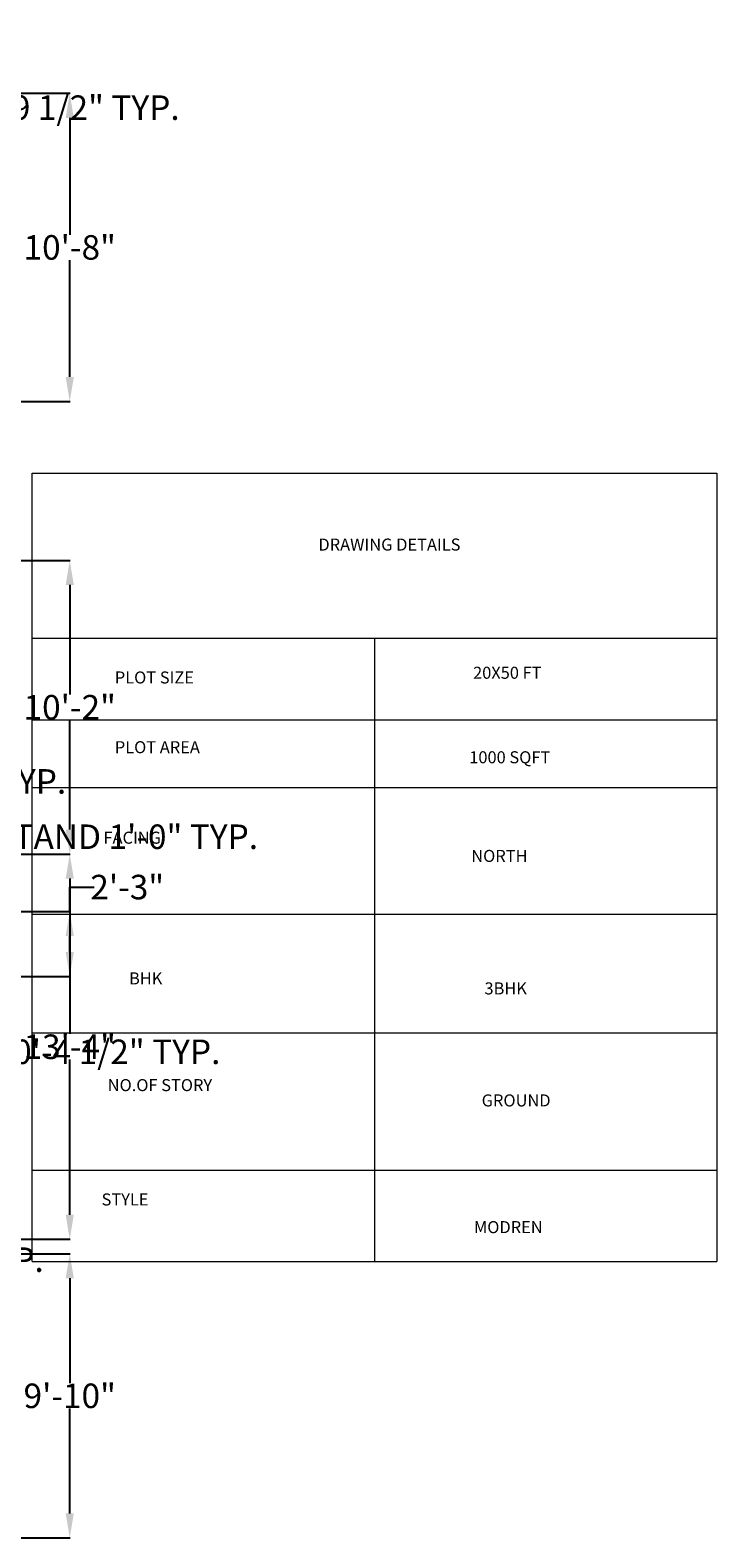
# Model space of a CAD drawing. Units: inches. Extents: x 1294 to 2470, y 659 to 1389.
# Tile 4 of 4: x 1714 to 2000, y 742 to 1368. Entities that reach past the tile are written whole.
import ezdxf

# ---------------------------------------------------------------- set-up
doc = ezdxf.new("R2010")
doc.units = ezdxf.units.IN
doc.header["$MEASUREMENT"] = 0
for name, color, linetype, lineweight in [('A-ANNO-DIMS', 2, 'Continuous', 18), ('A-ANNO-TEXT', 7, 'Continuous', 18), ('A-ANNO-TTLB', 7, 'Continuous', 18)]:
    doc.layers.add(name, color=color, linetype=linetype, lineweight=lineweight)
doc.styles.get("Standard").update_dxf_attribs({"font": 'arial.ttf'})
doc.dimstyles.get("Standard").update_dxf_attribs({"dimtxt": 10.18, "dimasz": 10.18, "dimexe": 0.18, "dimexo": 0.0625, "dimgap": 0.09, "dimtad": 0, "dimtih": 1, "dimtoh": 1, "dimdec": 0, "dimzin": 0, "dimdsep": 46, "dimlunit": 3, "dimtxsty": 'Standard', "dimcen": 0.09, "dimadec": 0, "dimazin": 0, "dimtfac": 1, "dimtdec": 0, "dimtofl": 0, "dimtmove": 0, "dimatfit": 3, "dimfxl": 1, "dimtolj": 1, "dimtzin": 0, "dimarcsym": 0})

# ---------------------------------------------------------------- blocks, each defined once
blk = doc.blocks.new('*D16')
at = {"layer": 'A-ANNO-DIMS', "color": 0, "lineweight": -2, "transparency": 16777216}
for p, q in [((1493.39, 862.72), (1493.39, 857.16)), ((1529.66, 862.72), (1529.66, 857.16)), ((1503.57, 857.34), (1519.48, 857.34)), ((1529.66, 857.34), (1539.84, 857.34))]:
    blk.add_line(p, q, dxfattribs=at)
at = {"layer": 'A-ANNO-DIMS', "color": 0, "transparency": 16777216}
for points in [[(1503.57, 859.04), (1503.57, 855.65), (1493.39, 857.34)], [(1519.48, 859.04), (1519.48, 855.65), (1529.66, 857.34)]]:
    blk.add_solid(points, dxfattribs=at)
at = {"layer": 'Defpoints', "color": 0, "transparency": 16777216}
for p in [(1493.39, 862.78), (1529.66, 862.78), (1529.66, 857.34)]:
    blk.add_point(p, dxfattribs=at)
at = {"layer": 'A-ANNO-DIMS', "color": 0, "transparency": 16777216, "insert": (1632.17, 857.34), "char_height": 10.18, "attachment_point": 5}
blk.add_mtext('\\A1;SWING DOOR 3\'-0 1/2" TYP.', dxfattribs=at)
blk = doc.blocks.new('*D19')
at = {"layer": 'A-ANNO-DIMS', "color": 0, "lineweight": -2, "transparency": 16777216}
for p, q in [((1640.66, 1063.72), (1640.66, 1055.8)), ((1646.66, 1063.72), (1646.66, 1055.8)), ((1630.48, 1055.98), (1620.3, 1055.98)), ((1656.84, 1055.98), (1667.02, 1055.98))]:
    blk.add_line(p, q, dxfattribs=at)
at = {"layer": 'A-ANNO-DIMS', "color": 0, "transparency": 16777216}
for points in [[(1630.48, 1057.68), (1630.48, 1054.29), (1640.66, 1055.98)], [(1656.84, 1057.68), (1656.84, 1054.29), (1646.66, 1055.98)]]:
    blk.add_solid(points, dxfattribs=at)
at = {"layer": 'Defpoints', "color": 0, "transparency": 16777216}
for p in [(1640.66, 1063.78), (1646.66, 1063.78), (1646.66, 1055.98)]:
    blk.add_point(p, dxfattribs=at)
at = {"layer": 'A-ANNO-DIMS', "color": 0, "transparency": 16777216, "insert": (1698.14, 1055.98), "char_height": 10.18, "attachment_point": 5}
blk.add_mtext('\\A1;0\'-6" TYP.', dxfattribs=at)
blk = doc.blocks.new('*D22')
at = {"layer": 'A-ANNO-DIMS', "color": 0, "lineweight": -2, "transparency": 16777216}
for p, q in [((1636.23, 933.49), (1636.23, 943.67)), ((1636.23, 943.67), (1646.41, 943.67)), ((1635.64, 923.31), (1636.41, 923.31)), ((1635.64, 918.98), (1636.41, 918.98)), ((1636.23, 908.8), (1636.23, 898.62))]:
    blk.add_line(p, q, dxfattribs=at)
at = {"layer": 'A-ANNO-DIMS', "color": 0, "transparency": 16777216}
for points in [[(1634.53, 933.49), (1637.92, 933.49), (1636.23, 923.31)], [(1634.53, 908.8), (1637.92, 908.8), (1636.23, 918.98)]]:
    blk.add_solid(points, dxfattribs=at)
at = {"layer": 'Defpoints', "color": 0, "transparency": 16777216}
for p in [(1635.58, 923.31), (1636.23, 923.31), (1635.58, 918.98)]:
    blk.add_point(p, dxfattribs=at)
at = {"layer": 'A-ANNO-DIMS', "color": 0, "transparency": 16777216, "insert": (1721.16, 943.67), "char_height": 10.18, "attachment_point": 5}
blk.add_mtext('\\A1;BURNER 0\'-4 1/2" TYP.', dxfattribs=at)
blk = doc.blocks.new('*D24')
at = {"layer": 'A-ANNO-DIMS', "color": 0, "lineweight": -2, "transparency": 16777216}
for p, q in [((1609.43, 1335.84), (1599.25, 1335.84)), ((1619.61, 1334.46), (1619.61, 1336.02)), ((1629.26, 1334.46), (1629.26, 1336.02)), ((1639.44, 1335.84), (1649.62, 1335.84))]:
    blk.add_line(p, q, dxfattribs=at)
at = {"layer": 'A-ANNO-DIMS', "color": 0, "transparency": 16777216}
for points in [[(1609.43, 1337.54), (1609.43, 1334.14), (1619.61, 1335.84)], [(1639.44, 1337.54), (1639.44, 1334.14), (1629.26, 1335.84)]]:
    blk.add_solid(points, dxfattribs=at)
at = {"layer": 'Defpoints', "color": 0, "transparency": 16777216}
for p in [(1619.61, 1334.39), (1629.26, 1335.84), (1629.26, 1334.39)]:
    blk.add_point(p, dxfattribs=at)
at = {"layer": 'A-ANNO-DIMS', "color": 0, "transparency": 16777216, "insert": (1713.71, 1335.84), "char_height": 10.18, "attachment_point": 5}
blk.add_mtext('\\A1;LAMP 0\'-9 1/2" TYP.', dxfattribs=at)
blk = doc.blocks.new('*D26')
at = {"layer": 'A-ANNO-DIMS', "color": 0, "lineweight": -2, "transparency": 16777216}
for p, q in [((1621.57, 1034.72), (1621.57, 1032.82)), ((1633.51, 1034.72), (1633.51, 1032.82)), ((1611.39, 1033), (1601.21, 1033)), ((1643.69, 1033), (1653.87, 1033))]:
    blk.add_line(p, q, dxfattribs=at)
at = {"layer": 'A-ANNO-DIMS', "color": 0, "transparency": 16777216}
for points in [[(1611.39, 1034.69), (1611.39, 1031.3), (1621.57, 1033)], [(1643.69, 1034.69), (1643.69, 1031.3), (1633.51, 1033)]]:
    blk.add_solid(points, dxfattribs=at)
at = {"layer": 'Defpoints', "color": 0, "transparency": 16777216}
for p in [(1621.57, 1034.79), (1633.51, 1034.79), (1633.51, 1033)]:
    blk.add_point(p, dxfattribs=at)
at = {"layer": 'A-ANNO-DIMS', "color": 0, "transparency": 16777216, "insert": (1732.93, 1033), "char_height": 10.18, "attachment_point": 5}
blk.add_mtext('\\A1;NIGHTSTAND 1\'-0" TYP.', dxfattribs=at)
blk = doc.blocks.new('*D37')
at = {"layer": 'A-ANNO-DIMS', "color": 0, "lineweight": -2, "transparency": 16777216}
for p, q in [((1640.72, 859.78), (1730.86, 859.78)), ((1730.68, 849.6), (1730.68, 806.07)), ((1730.68, 751.96), (1730.68, 795.5)), ((1646.72, 741.78), (1730.86, 741.78))]:
    blk.add_line(p, q, dxfattribs=at)
at = {"layer": 'A-ANNO-DIMS', "color": 0, "transparency": 16777216}
for points in [[(1728.99, 849.6), (1732.38, 849.6), (1730.68, 859.78)], [(1728.99, 751.96), (1732.38, 751.96), (1730.68, 741.78)]]:
    blk.add_solid(points, dxfattribs=at)
at = {"layer": 'Defpoints', "color": 0, "transparency": 16777216}
for p in [(1640.66, 859.78), (1730.68, 859.78), (1646.66, 741.78)]:
    blk.add_point(p, dxfattribs=at)
at = {"layer": 'A-ANNO-DIMS', "color": 0, "transparency": 16777216, "insert": (1730.68, 800.78), "char_height": 10.18, "attachment_point": 5}
blk.add_mtext('\\A1;9\'-10"', dxfattribs=at)
blk = doc.blocks.new('*D38')
at = {"layer": 'A-ANNO-DIMS', "color": 0, "lineweight": -2, "transparency": 16777216}
for p, q in [((1640.72, 1025.78), (1730.86, 1025.78)), ((1730.68, 1015.6), (1730.68, 951.07)), ((1730.68, 875.96), (1730.68, 940.49)), ((1640.72, 865.78), (1730.86, 865.78))]:
    blk.add_line(p, q, dxfattribs=at)
at = {"layer": 'A-ANNO-DIMS', "color": 0, "transparency": 16777216}
for points in [[(1728.99, 1015.6), (1732.38, 1015.6), (1730.68, 1025.78)], [(1728.99, 875.96), (1732.38, 875.96), (1730.68, 865.78)]]:
    blk.add_solid(points, dxfattribs=at)
at = {"layer": 'Defpoints', "color": 0, "transparency": 16777216}
for p in [(1640.66, 1025.78), (1730.68, 1025.78), (1640.66, 865.78)]:
    blk.add_point(p, dxfattribs=at)
at = {"layer": 'A-ANNO-DIMS', "color": 0, "transparency": 16777216, "insert": (1730.68, 945.78), "char_height": 10.18, "attachment_point": 5}
blk.add_mtext('\\A1;13\'-4"', dxfattribs=at)
blk = doc.blocks.new('*D39')
at = {"layer": 'A-ANNO-DIMS', "color": 0, "lineweight": -2, "transparency": 16777216}
for p, q in [((1640.72, 1147.78), (1730.86, 1147.78)), ((1730.68, 1137.6), (1730.68, 1092.07)), ((1730.68, 1035.96), (1730.68, 1081.5)), ((1640.72, 1025.78), (1730.86, 1025.78))]:
    blk.add_line(p, q, dxfattribs=at)
at = {"layer": 'A-ANNO-DIMS', "color": 0, "transparency": 16777216}
for points in [[(1728.99, 1137.6), (1732.38, 1137.6), (1730.68, 1147.78)], [(1728.99, 1035.96), (1732.38, 1035.96), (1730.68, 1025.78)]]:
    blk.add_solid(points, dxfattribs=at)
at = {"layer": 'Defpoints', "color": 0, "transparency": 16777216}
for p in [(1640.66, 1147.78), (1730.68, 1147.78), (1640.66, 1025.78)]:
    blk.add_point(p, dxfattribs=at)
at = {"layer": 'A-ANNO-DIMS', "color": 0, "transparency": 16777216, "insert": (1730.68, 1086.78), "char_height": 10.18, "attachment_point": 5}
blk.add_mtext('\\A1;10\'-2"', dxfattribs=at)
blk = doc.blocks.new('*D41')
at = {"layer": 'A-ANNO-DIMS', "color": 0, "lineweight": -2, "transparency": 16777216}
for p, q in [((1646.72, 1341.78), (1730.86, 1341.78)), ((1730.68, 1331.6), (1730.68, 1283.07)), ((1730.68, 1223.96), (1730.68, 1272.5)), ((1640.72, 1213.78), (1730.86, 1213.78))]:
    blk.add_line(p, q, dxfattribs=at)
at = {"layer": 'A-ANNO-DIMS', "color": 0, "transparency": 16777216}
for points in [[(1728.99, 1331.6), (1732.38, 1331.6), (1730.68, 1341.78)], [(1728.99, 1223.96), (1732.38, 1223.96), (1730.68, 1213.78)]]:
    blk.add_solid(points, dxfattribs=at)
at = {"layer": 'Defpoints', "color": 0, "transparency": 16777216}
for p in [(1646.66, 1341.78), (1730.68, 1341.78), (1640.66, 1213.78)]:
    blk.add_point(p, dxfattribs=at)
at = {"layer": 'A-ANNO-DIMS', "color": 0, "transparency": 16777216, "insert": (1730.68, 1277.78), "char_height": 10.18, "attachment_point": 5}
blk.add_mtext('\\A1;10\'-8"', dxfattribs=at)
blk = doc.blocks.new('*D51')
at = {"layer": 'A-ANNO-DIMS', "color": 0, "lineweight": -2, "transparency": 16777216}
for p, q in [((1730.68, 1001.91), (1730.68, 1012.09)), ((1730.68, 1012.09), (1740.86, 1012.09)), ((1618.71, 1001.91), (1730.86, 1001.91)), ((1730.68, 985.08), (1730.68, 991.73)), ((1618.71, 974.9), (1730.86, 974.9))]:
    blk.add_line(p, q, dxfattribs=at)
at = {"layer": 'A-ANNO-DIMS', "color": 0, "transparency": 16777216}
for points in [[(1728.99, 991.73), (1732.38, 991.73), (1730.68, 1001.91)], [(1728.99, 985.08), (1732.38, 985.08), (1730.68, 974.9)]]:
    blk.add_solid(points, dxfattribs=at)
at = {"layer": 'Defpoints', "color": 0, "transparency": 16777216}
for p in [(1618.65, 1001.91), (1730.68, 1001.91), (1618.65, 974.9)]:
    blk.add_point(p, dxfattribs=at)
at = {"layer": 'A-ANNO-DIMS', "color": 0, "transparency": 16777216, "insert": (1754.57, 1012.09), "char_height": 10.18, "attachment_point": 5}
blk.add_mtext('\\A1;2\'-3"', dxfattribs=at)

msp = doc.modelspace()

# ---------------------------------------------------------------- linework, layer by layer
at = {"layer": 'A-ANNO-TTLB'}
for p, q in [((1715.1, 1115.54), (1999.56, 1115.54)), ((1857.33, 1115.54), (1857.33, 856.55)), ((1715.1, 1081.59), (1999.56, 1081.59)), ((1715.1, 1053.51), (1999.56, 1053.51)), ((1715.1, 1000.84), (1999.56, 1000.84)), ((1715.1, 951.59), (1999.56, 951.59)), ((1715.1, 894.56), (1999.56, 894.56)), ((1715.1, 856.55), (1999.56, 856.55))]:
    msp.add_line(p, q, dxfattribs=at)
msp.add_lwpolyline([(1715.1, 856.55), (1715.1, 1183.99), (1715.1, 1183.99), (1999.56, 1183.99), (1999.56, 1183.99), (1999.56, 856.55)], dxfattribs=at)

# ---------------------------------------------------------------- texts
at = {"layer": 'A-ANNO-TEXT', "char_height": 5, "attachment_point": 1}
for s, insert in [('DRAWING DETAILS', (1833.99, 1156.85)), ('20X50 FT', (1898.27, 1103.61)), ('PLOT SIZE', (1749.41, 1101.65)), ('PLOT AREA', (1749.41, 1072.69)), ('1000 SQFT', (1896.69, 1068.5)), ('FACING', (1744.7, 1035.11)), ('NORTH', (1897.51, 1027.53)), ('BHK', (1755.32, 976.66)), ('3BHK', (1903, 972.5)), ('NO.OF STORY', (1746.45, 932.33)), ('GROUND', (1901.84, 925.97)), ('STYLE', (1743.91, 884.84)), ('MODREN', (1898.62, 873.34))]:
    msp.add_mtext_dynamic_manual_height_columns(s, width=162.3199, gutter_width=1, heights=[0], dxfattribs=dict(at, insert=insert))

# ---------------------------------------------------------------- dimensions: what is measured, and where the dimension line sits
at = {"layer": 'A-ANNO-DIMS'}
for base, p1, p2, text, picture, middle in [((1629.263, 1335.8411), (1619.6124, 1334.3935), (1629.263, 1334.3935), 'LAMP <> TYP.', '*D24', (1713.713, 1335.8411)), ((1646.66, 1055.98), (1640.66, 1063.78), (1646.66, 1063.78), '<> TYP.', '*D19', (1698.14, 1055.98)), ((1633.51, 1033), (1621.57, 1034.79), (1633.51, 1034.79), 'NIGHTSTAND <> TYP.', '*D26', (1732.93, 1033)), ((1529.66, 857.34), (1493.39, 862.78), (1529.66, 862.78), 'SWING DOOR <> TYP.', '*D16', (1632.17, 857.34))]:
    dim = msp.add_linear_dim(base=base, p1=p1, p2=p2, text=text, dimstyle='Standard', override={"dimdec": 1, "dimlfac": 1, "dimrnd": 0, "dimzin": 1, "dimdsep": 46, "dimlunit": 4, "dimfrac": 2}, dxfattribs=at)
    dim.commit()
    dim.dimension.update_dxf_attribs({"geometry": picture, "text_midpoint": middle})
for base, p1, p2, picture, middle in [((1730.68, 1341.78), (1640.66, 1213.78), (1646.66, 1341.78), '*D41', (1730.68, 1277.78)), ((1730.68, 1147.78), (1640.66, 1025.78), (1640.66, 1147.78), '*D39', (1730.68, 1086.78)), ((1730.68, 1025.78), (1640.66, 865.78), (1640.66, 1025.78), '*D38', (1730.68, 945.78)), ((1730.68, 1001.91), (1618.65, 974.9), (1618.65, 1001.91), '*D51', (1754.57, 1012.09)), ((1730.68, 859.78), (1646.66, 741.78), (1640.66, 859.78), '*D37', (1730.68, 800.78))]:
    dim = msp.add_linear_dim(base=base, p1=p1, p2=p2, angle=90, dimstyle='Standard', override={"dimdec": 1, "dimlfac": 1, "dimrnd": 0, "dimzin": 1, "dimdsep": 46, "dimlunit": 4, "dimfrac": 2}, dxfattribs=at)
    dim.commit()
    dim.dimension.update_dxf_attribs({"geometry": picture, "text_midpoint": middle})
dim = msp.add_linear_dim(base=(1636.23, 923.31), p1=(1635.58, 918.98), p2=(1635.58, 923.31), angle=90, text='BURNER <> TYP.', dimstyle='Standard', override={"dimdec": 1, "dimlfac": 1, "dimrnd": 0, "dimzin": 1, "dimdsep": 46, "dimlunit": 4, "dimfrac": 2}, dxfattribs=at)
dim.commit()
dim.dimension.update_dxf_attribs({"geometry": '*D22', "text_midpoint": (1721.16, 943.67)})

doc.saveas('drawing.dxf')
